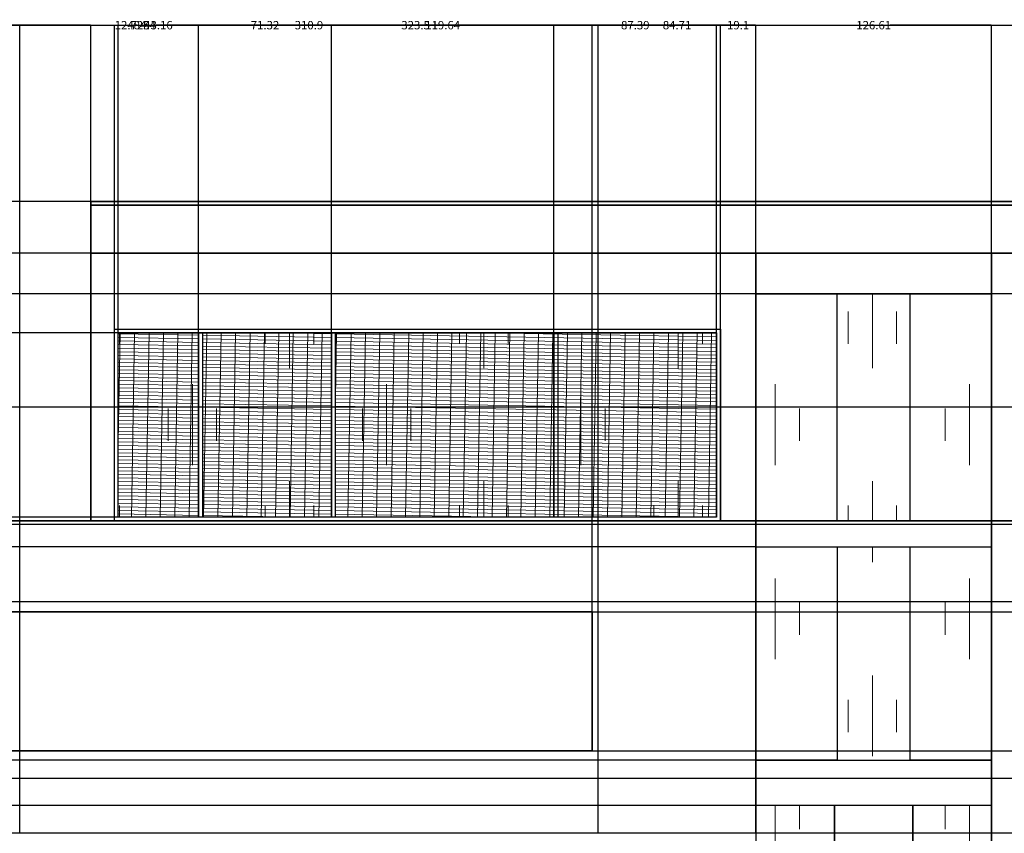
# Model space of a CAD drawing. Units: inches. Extents: x -1308 to 780, y 304 to 1023.
# Tile 4 of 7: x -667 to -138, y 585 to 1023. Entities that reach past the tile are written whole.
import ezdxf

# ---------------------------------------------------------------- set-up
doc = ezdxf.new("R2010")
doc.units = ezdxf.units.IN
doc.header["$MEASUREMENT"] = 0
for name, color, linetype, lineweight in [('A-ANNO-DIMS', 2, 'Continuous', 18), ('A-ELEV', 7, 'Continuous', 35), ('A-ELEV-PATT', 8, 'Continuous', 13), ('A-GLAZ', 4, 'Continuous', 25)]:
    doc.layers.add(name, color=color, linetype=linetype, lineweight=lineweight)
doc.styles.get("Standard").update_dxf_attribs({"font": 'arial.ttf'})
doc.dimstyles.get("Standard").update_dxf_attribs({"dimtxt": 4.5, "dimasz": 0.18, "dimexe": 0.18, "dimexo": 0.0625, "dimgap": 0.09, "dimtad": 0, "dimtih": 1, "dimtoh": 1, "dimdec": 4, "dimzin": 0, "dimdsep": 46, "dimlunit": 4, "dimtxsty": 'Standard', "dimcen": 0.09, "dimadec": 0, "dimazin": 0, "dimtfac": 1, "dimtdec": 4, "dimtofl": 0, "dimtmove": 0, "dimatfit": 3, "dimfxl": 1, "dimtolj": 1, "dimtzin": 0, "dimarcsym": 0})

# ---------------------------------------------------------------- blocks, each defined once
blk = doc.blocks.new('*D6')
at = {"layer": 'A-ANNO-DIMS', "color": 0, "lineweight": -2, "transparency": 16777216}
for p, q in [((-666.95, 585.1), (-666.95, 1019.77)), ((-666.77, 1019.59), (-519.19, 1019.59)), ((-356.24, 1019.59), (-503.82, 1019.59)), ((-356.06, 585.1), (-356.06, 1019.77))]:
    blk.add_line(p, q, dxfattribs=at)
at = {"layer": 'A-ANNO-DIMS', "color": 0, "transparency": 16777216}
for points in [[(-666.77, 1019.62), (-666.77, 1019.56), (-666.95, 1019.59)], [(-356.24, 1019.62), (-356.24, 1019.56), (-356.06, 1019.59)]]:
    blk.add_solid(points, dxfattribs=at)
at = {"layer": 'Defpoints', "color": 0, "transparency": 16777216}
for p in [(-356.06, 1019.59), (-666.95, 585.04), (-356.06, 585.04)]:
    blk.add_point(p, dxfattribs=at)
at = {"layer": 'A-ANNO-DIMS', "color": 0, "transparency": 16777216, "insert": (-511.5, 1019.59), "char_height": 4.5, "attachment_point": 5}
blk.add_mtext('\\A1;310.9', dxfattribs=at)
blk = doc.blocks.new('*D7')
at = {"layer": 'A-ANNO-DIMS', "color": 0, "lineweight": -2, "transparency": 16777216}
for p, q in [((-356.06, 585.1), (-356.06, 1019.77)), ((-355.88, 1019.59), (-320.95, 1019.59)), ((-271.53, 1019.59), (-306.45, 1019.59)), ((-271.35, 585.1), (-271.35, 1019.77))]:
    blk.add_line(p, q, dxfattribs=at)
at = {"layer": 'A-ANNO-DIMS', "color": 0, "transparency": 16777216}
for points in [[(-355.88, 1019.62), (-355.88, 1019.56), (-356.06, 1019.59)], [(-271.53, 1019.62), (-271.53, 1019.56), (-271.35, 1019.59)]]:
    blk.add_solid(points, dxfattribs=at)
at = {"layer": 'Defpoints', "color": 0, "transparency": 16777216}
for p in [(-271.35, 1019.59), (-356.06, 585.04), (-271.35, 585.04)]:
    blk.add_point(p, dxfattribs=at)
at = {"layer": 'A-ANNO-DIMS', "color": 0, "transparency": 16777216, "insert": (-313.7, 1019.59), "char_height": 4.5, "attachment_point": 5}
blk.add_mtext('\\A1;84.71', dxfattribs=at)
blk = doc.blocks.new('*D8')
at = {"layer": 'A-ANNO-DIMS', "color": 0, "lineweight": -2, "transparency": 16777216}
for p, q in [((-271.35, 585.1), (-271.35, 1019.77)), ((-271.17, 1019.59), (-216.82, 1019.59)), ((-144.91, 1019.59), (-199.25, 1019.59)), ((-144.73, 585.1), (-144.73, 1019.77))]:
    blk.add_line(p, q, dxfattribs=at)
at = {"layer": 'A-ANNO-DIMS', "color": 0, "transparency": 16777216}
for points in [[(-271.17, 1019.62), (-271.17, 1019.56), (-271.35, 1019.59)], [(-144.91, 1019.62), (-144.91, 1019.56), (-144.73, 1019.59)]]:
    blk.add_solid(points, dxfattribs=at)
at = {"layer": 'Defpoints', "color": 0, "transparency": 16777216}
for p in [(-144.73, 1019.59), (-271.35, 585.04), (-144.73, 585.04)]:
    blk.add_point(p, dxfattribs=at)
at = {"layer": 'A-ANNO-DIMS', "color": 0, "transparency": 16777216, "insert": (-208.04, 1019.59), "char_height": 4.5, "attachment_point": 5}
blk.add_mtext('\\A1;126.61', dxfattribs=at)
blk = doc.blocks.new('*D17')
at = {"layer": 'A-ANNO-DIMS', "color": 0, "lineweight": -2, "transparency": 16777216}
for p, q in [((-843.6, 753.1), (-843.6, 1019.77)), ((-843.42, 1019.59), (-743.87, 1019.59)), ((-628.86, 1019.59), (-728.41, 1019.59)), ((-628.68, 753.1), (-628.68, 1019.77))]:
    blk.add_line(p, q, dxfattribs=at)
at = {"layer": 'A-ANNO-DIMS', "color": 0, "transparency": 16777216}
for points in [[(-843.42, 1019.62), (-843.42, 1019.56), (-843.6, 1019.59)], [(-628.86, 1019.62), (-628.86, 1019.56), (-628.68, 1019.59)]]:
    blk.add_solid(points, dxfattribs=at)
at = {"layer": 'Defpoints', "color": 0, "transparency": 16777216}
for p in [(-628.68, 1019.59), (-843.6, 753.04), (-628.68, 753.04)]:
    blk.add_point(p, dxfattribs=at)
at = {"layer": 'A-ANNO-DIMS', "color": 0, "transparency": 16777216, "insert": (-736.14, 1019.59), "char_height": 4.5, "attachment_point": 5}
blk.add_mtext('\\A1;214.9', dxfattribs=at)
blk = doc.blocks.new('*D18')
at = {"layer": 'A-ANNO-DIMS', "color": 0, "lineweight": -2, "transparency": 16777216}
for p, q in [((-628.68, 924.9), (-628.68, 1019.77)), ((-628.5, 1019.59), (-60.08, 1019.59)), ((526.78, 1019.59), (-41.64, 1019.59)), ((526.96, 924.9), (526.96, 1019.77))]:
    blk.add_line(p, q, dxfattribs=at)
at = {"layer": 'A-ANNO-DIMS', "color": 0, "transparency": 16777216}
for points in [[(-628.5, 1019.62), (-628.5, 1019.56), (-628.68, 1019.59)], [(526.78, 1019.62), (526.78, 1019.56), (526.96, 1019.59)]]:
    blk.add_solid(points, dxfattribs=at)
at = {"layer": 'Defpoints', "color": 0, "transparency": 16777216}
for p in [(526.96, 1019.59), (-628.68, 924.84), (526.96, 924.84)]:
    blk.add_point(p, dxfattribs=at)
at = {"layer": 'A-ANNO-DIMS', "color": 0, "transparency": 16777216, "insert": (-50.86, 1019.59), "char_height": 4.5, "attachment_point": 5}
blk.add_mtext('\\A1;1155.6', dxfattribs=at)
blk = doc.blocks.new('*D20')
at = {"layer": 'A-ANNO-DIMS', "color": 0, "lineweight": -2, "transparency": 16777216}
for p, q in [((-615.96, 856.16), (-615.96, 1019.77)), ((-615.78, 1019.59), (-461.9, 1019.59)), ((-292.63, 1019.59), (-446.5, 1019.59)), ((-292.45, 854.16), (-292.45, 1019.77))]:
    blk.add_line(p, q, dxfattribs=at)
at = {"layer": 'A-ANNO-DIMS', "color": 0, "transparency": 16777216}
for points in [[(-615.78, 1019.62), (-615.78, 1019.56), (-615.96, 1019.59)], [(-292.63, 1019.62), (-292.63, 1019.56), (-292.45, 1019.59)]]:
    blk.add_solid(points, dxfattribs=at)
at = {"layer": 'Defpoints', "color": 0, "transparency": 16777216}
for p in [(-292.45, 1019.59), (-615.96, 856.09), (-292.45, 854.09)]:
    blk.add_point(p, dxfattribs=at)
at = {"layer": 'A-ANNO-DIMS', "color": 0, "transparency": 16777216, "insert": (-454.2, 1019.59), "char_height": 4.5, "attachment_point": 5}
blk.add_mtext('\\A1;323.5', dxfattribs=at)
blk = doc.blocks.new('*D21')
at = {"layer": 'A-ANNO-DIMS', "color": 0, "lineweight": -2, "transparency": 16777216}
for p, q in [((-628.68, 753.1), (-628.68, 1019.77)), ((-628.5, 1019.59), (-616.14, 1019.59)), ((-615.96, 753.1), (-615.96, 1019.77)), ((-615.96, 1019.59), (-615.78, 1019.59))]:
    blk.add_line(p, q, dxfattribs=at)
at = {"layer": 'A-ANNO-DIMS', "color": 0, "transparency": 16777216}
for points in [[(-628.5, 1019.62), (-628.5, 1019.56), (-628.68, 1019.59)], [(-616.14, 1019.62), (-616.14, 1019.56), (-615.96, 1019.59)]]:
    blk.add_solid(points, dxfattribs=at)
at = {"layer": 'Defpoints', "color": 0, "transparency": 16777216}
for p in [(-615.96, 1019.59), (-628.68, 753.04), (-615.96, 753.04)]:
    blk.add_point(p, dxfattribs=at)
at = {"layer": 'A-ANNO-DIMS', "color": 0, "transparency": 16777216, "insert": (-606.54, 1019.59), "char_height": 4.5, "attachment_point": 5}
blk.add_mtext('\\A1;12.725', dxfattribs=at)
blk = doc.blocks.new('*D22')
at = {"layer": 'A-ANNO-DIMS', "color": 0, "lineweight": -2, "transparency": 16777216}
for p, q in [((-290.45, 753.1), (-290.45, 1019.77)), ((-290.27, 1019.59), (-286.18, 1019.59)), ((-271.53, 1019.59), (-275.61, 1019.59)), ((-271.35, 753.1), (-271.35, 1019.77))]:
    blk.add_line(p, q, dxfattribs=at)
at = {"layer": 'A-ANNO-DIMS', "color": 0, "transparency": 16777216}
for points in [[(-290.27, 1019.62), (-290.27, 1019.56), (-290.45, 1019.59)], [(-271.53, 1019.62), (-271.53, 1019.56), (-271.35, 1019.59)]]:
    blk.add_solid(points, dxfattribs=at)
at = {"layer": 'Defpoints', "color": 0, "transparency": 16777216}
for p in [(-271.35, 1019.59), (-290.45, 753.04), (-271.35, 753.04)]:
    blk.add_point(p, dxfattribs=at)
at = {"layer": 'A-ANNO-DIMS', "color": 0, "transparency": 16777216, "insert": (-280.9, 1019.59), "char_height": 4.5, "attachment_point": 5}
blk.add_mtext('\\A1;19.1', dxfattribs=at)
blk = doc.blocks.new('*D23')
at = {"layer": 'A-ANNO-DIMS', "color": 0, "lineweight": -2, "transparency": 16777216}
for p, q in [((-613.96, 755.1), (-613.96, 1019.77)), ((-613.78, 1019.59), (-600.15, 1019.59)), ((-570.98, 1019.59), (-584.6, 1019.59)), ((-570.8, 755.1), (-570.8, 1019.77))]:
    blk.add_line(p, q, dxfattribs=at)
at = {"layer": 'A-ANNO-DIMS', "color": 0, "transparency": 16777216}
for points in [[(-613.78, 1019.62), (-613.78, 1019.56), (-613.96, 1019.59)], [(-570.98, 1019.62), (-570.98, 1019.56), (-570.8, 1019.59)]]:
    blk.add_solid(points, dxfattribs=at)
at = {"layer": 'Defpoints', "color": 0, "transparency": 16777216}
for p in [(-570.8, 1019.59), (-613.96, 755.04), (-570.8, 755.04)]:
    blk.add_point(p, dxfattribs=at)
at = {"layer": 'A-ANNO-DIMS', "color": 0, "transparency": 16777216, "insert": (-592.38, 1019.59), "char_height": 4.5, "attachment_point": 5}
blk.add_mtext('\\A1;43.16', dxfattribs=at)
blk = doc.blocks.new('*D24')
at = {"layer": 'A-ANNO-DIMS', "color": 0, "lineweight": -2, "transparency": 16777216}
for p, q in [((-570.8, 755.1), (-570.8, 1019.77)), ((-570.62, 1019.59), (-542.78, 1019.59)), ((-499.65, 1019.59), (-527.49, 1019.59)), ((-499.47, 755.1), (-499.47, 1019.77))]:
    blk.add_line(p, q, dxfattribs=at)
at = {"layer": 'A-ANNO-DIMS', "color": 0, "transparency": 16777216}
for points in [[(-570.62, 1019.62), (-570.62, 1019.56), (-570.8, 1019.59)], [(-499.65, 1019.62), (-499.65, 1019.56), (-499.47, 1019.59)]]:
    blk.add_solid(points, dxfattribs=at)
at = {"layer": 'Defpoints', "color": 0, "transparency": 16777216}
for p in [(-499.47, 1019.59), (-570.8, 755.04), (-499.47, 755.04)]:
    blk.add_point(p, dxfattribs=at)
at = {"layer": 'A-ANNO-DIMS', "color": 0, "transparency": 16777216, "insert": (-535.13, 1019.59), "char_height": 4.5, "attachment_point": 5}
blk.add_mtext('\\A1;71.32', dxfattribs=at)
blk = doc.blocks.new('*D25')
at = {"layer": 'A-ANNO-DIMS', "color": 0, "lineweight": -2, "transparency": 16777216}
for p, q in [((-499.47, 755.1), (-499.47, 1019.77)), ((-499.29, 1019.59), (-448.86, 1019.59)), ((-380.02, 1019.59), (-430.45, 1019.59)), ((-379.84, 755.1), (-379.84, 1019.77))]:
    blk.add_line(p, q, dxfattribs=at)
at = {"layer": 'A-ANNO-DIMS', "color": 0, "transparency": 16777216}
for points in [[(-499.29, 1019.62), (-499.29, 1019.56), (-499.47, 1019.59)], [(-380.02, 1019.62), (-380.02, 1019.56), (-379.84, 1019.59)]]:
    blk.add_solid(points, dxfattribs=at)
at = {"layer": 'Defpoints', "color": 0, "transparency": 16777216}
for p in [(-379.84, 1019.59), (-499.47, 755.04), (-379.84, 755.04)]:
    blk.add_point(p, dxfattribs=at)
at = {"layer": 'A-ANNO-DIMS', "color": 0, "transparency": 16777216, "insert": (-439.65, 1019.59), "char_height": 4.5, "attachment_point": 5}
blk.add_mtext('\\A1;119.64', dxfattribs=at)
blk = doc.blocks.new('*D26')
at = {"layer": 'A-ANNO-DIMS', "color": 0, "lineweight": -2, "transparency": 16777216}
for p, q in [((-379.84, 755.1), (-379.84, 1019.77)), ((-379.66, 1019.59), (-343.83, 1019.59)), ((-292.63, 1019.59), (-328.45, 1019.59)), ((-292.45, 755.1), (-292.45, 1019.77))]:
    blk.add_line(p, q, dxfattribs=at)
at = {"layer": 'A-ANNO-DIMS', "color": 0, "transparency": 16777216}
for points in [[(-379.66, 1019.62), (-379.66, 1019.56), (-379.84, 1019.59)], [(-292.63, 1019.62), (-292.63, 1019.56), (-292.45, 1019.59)]]:
    blk.add_solid(points, dxfattribs=at)
at = {"layer": 'Defpoints', "color": 0, "transparency": 16777216}
for p in [(-292.45, 1019.59), (-379.84, 755.04), (-292.45, 755.04)]:
    blk.add_point(p, dxfattribs=at)
at = {"layer": 'A-ANNO-DIMS', "color": 0, "transparency": 16777216, "insert": (-336.14, 1019.59), "char_height": 4.5, "attachment_point": 5}
blk.add_mtext('\\A1;87.39', dxfattribs=at)
blk = doc.blocks.new('*D27')
at = {"layer": 'A-ANNO-DIMS', "color": 0, "lineweight": -2, "transparency": 16777216}
for p, q in [((-144.73, 753.1), (-144.73, 1019.77)), ((-144.55, 1019.59), (-112.53, 1019.59)), ((-65.19, 1019.59), (-97.21, 1019.59)), ((-65.01, 751.1), (-65.01, 1019.77))]:
    blk.add_line(p, q, dxfattribs=at)
at = {"layer": 'A-ANNO-DIMS', "color": 0, "transparency": 16777216}
for points in [[(-144.55, 1019.62), (-144.55, 1019.56), (-144.73, 1019.59)], [(-65.19, 1019.62), (-65.19, 1019.56), (-65.01, 1019.59)]]:
    blk.add_solid(points, dxfattribs=at)
at = {"layer": 'Defpoints', "color": 0, "transparency": 16777216}
for p in [(-65.01, 1019.59), (-144.73, 753.04), (-65.01, 751.04)]:
    blk.add_point(p, dxfattribs=at)
at = {"layer": 'A-ANNO-DIMS', "color": 0, "transparency": 16777216, "insert": (-104.87, 1019.59), "char_height": 4.5, "attachment_point": 5}
blk.add_mtext('\\A1;79.73', dxfattribs=at)
blk = doc.blocks.new('*D45')
at = {"layer": 'A-ANNO-DIMS', "color": 0, "lineweight": -2, "transparency": 16777216}
for p, q in [((-25.86, 614.44), (-25.86, 307.09)), ((-144.73, 584.98), (-144.73, 307.09)), ((-144.55, 307.27), (-94.52, 307.27)), ((-26.04, 307.27), (-76.07, 307.27))]:
    blk.add_line(p, q, dxfattribs=at)
at = {"layer": 'A-ANNO-DIMS', "color": 0, "transparency": 16777216}
for points in [[(-144.55, 307.3), (-144.55, 307.24), (-144.73, 307.27)], [(-26.04, 307.3), (-26.04, 307.24), (-25.86, 307.27)]]:
    blk.add_solid(points, dxfattribs=at)
at = {"layer": 'Defpoints', "color": 0, "transparency": 16777216}
for p in [(-25.86, 614.51), (-144.73, 585.04), (-25.86, 307.27)]:
    blk.add_point(p, dxfattribs=at)
at = {"layer": 'A-ANNO-DIMS', "color": 0, "transparency": 16777216, "insert": (-85.3, 307.27), "char_height": 4.5, "attachment_point": 5}
blk.add_mtext('\\A1;118.88', dxfattribs=at)
blk = doc.blocks.new('*D48')
at = {"layer": 'A-ANNO-DIMS', "color": 0, "lineweight": -2, "transparency": 16777216}
for p, q in [((-843.6, 704.15), (-843.6, 1019.77)), ((-843.42, 1019.59), (-609.19, 1019.59)), ((-359.42, 1019.59), (-593.66, 1019.59)), ((-359.24, 704.15), (-359.24, 1019.77))]:
    blk.add_line(p, q, dxfattribs=at)
at = {"layer": 'A-ANNO-DIMS', "color": 0, "transparency": 16777216}
for points in [[(-843.42, 1019.62), (-843.42, 1019.56), (-843.6, 1019.59)], [(-359.42, 1019.62), (-359.42, 1019.56), (-359.24, 1019.59)]]:
    blk.add_solid(points, dxfattribs=at)
at = {"layer": 'Defpoints', "color": 0, "transparency": 16777216}
for p in [(-359.24, 1019.59), (-843.6, 704.09), (-359.24, 704.09)]:
    blk.add_point(p, dxfattribs=at)
at = {"layer": 'A-ANNO-DIMS', "color": 0, "transparency": 16777216, "insert": (-601.42, 1019.59), "char_height": 4.5, "attachment_point": 5}
blk.add_mtext('\\A1;484.4', dxfattribs=at)
blk = doc.blocks.new('*D57')
at = {"layer": 'A-ANNO-DIMS', "color": 0, "lineweight": -2, "transparency": 16777216}
for p, q in [((-628.74, 924.84), (-1298.45, 924.84)), ((-1298.27, 924.66), (-1298.27, 665.82)), ((-1298.27, 402.2), (-1298.27, 661.04)), ((-1203.58, 402.02), (-1298.45, 402.02))]:
    blk.add_line(p, q, dxfattribs=at)
at = {"layer": 'A-ANNO-DIMS', "color": 0, "transparency": 16777216}
for points in [[(-1298.3, 924.66), (-1298.24, 924.66), (-1298.27, 924.84)], [(-1298.3, 402.2), (-1298.24, 402.2), (-1298.27, 402.02)]]:
    blk.add_solid(points, dxfattribs=at)
at = {"layer": 'Defpoints', "color": 0, "transparency": 16777216}
for p in [(-1298.27, 924.84), (-628.68, 924.84), (-1203.52, 402.02)]:
    blk.add_point(p, dxfattribs=at)
at = {"layer": 'A-ANNO-DIMS', "color": 0, "transparency": 16777216, "insert": (-1298.27, 663.43), "char_height": 4.5, "attachment_point": 5}
blk.add_mtext('\\A1;522.8', dxfattribs=at)
blk = doc.blocks.new('*D63')
at = {"layer": 'A-ANNO-DIMS', "color": 0, "lineweight": -2, "transparency": 16777216}
for p, q in [((-843.54, 629.44), (771.09, 629.44)), ((770.91, 629.26), (770.91, 518.12)), ((770.91, 402.2), (770.91, 513.34)), ((-843.54, 402.02), (771.09, 402.02))]:
    blk.add_line(p, q, dxfattribs=at)
at = {"layer": 'A-ANNO-DIMS', "color": 0, "transparency": 16777216}
for points in [[(770.88, 629.26), (770.94, 629.26), (770.91, 629.44)], [(770.88, 402.2), (770.94, 402.2), (770.91, 402.02)]]:
    blk.add_solid(points, dxfattribs=at)
at = {"layer": 'Defpoints', "color": 0, "transparency": 16777216}
for p in [(-843.6, 629.44), (770.91, 629.44), (-843.6, 402.02)]:
    blk.add_point(p, dxfattribs=at)
at = {"layer": 'A-ANNO-DIMS', "color": 0, "transparency": 16777216, "insert": (770.91, 515.73), "char_height": 4.5, "attachment_point": 5}
blk.add_mtext('\\A1;227.43', dxfattribs=at)
blk = doc.blocks.new('*D64')
at = {"layer": 'A-ANNO-DIMS', "color": 0, "lineweight": -2, "transparency": 16777216}
for p, q in [((-843.54, 704.09), (771.09, 704.09)), ((770.91, 703.91), (770.91, 669.15)), ((770.91, 629.62), (770.91, 664.38)), ((-843.54, 629.44), (771.09, 629.44))]:
    blk.add_line(p, q, dxfattribs=at)
at = {"layer": 'A-ANNO-DIMS', "color": 0, "transparency": 16777216}
for points in [[(770.88, 703.91), (770.94, 703.91), (770.91, 704.09)], [(770.88, 629.62), (770.94, 629.62), (770.91, 629.44)]]:
    blk.add_solid(points, dxfattribs=at)
at = {"layer": 'Defpoints', "color": 0, "transparency": 16777216}
for p in [(-843.6, 704.09), (770.91, 704.09), (-843.6, 629.44)]:
    blk.add_point(p, dxfattribs=at)
at = {"layer": 'A-ANNO-DIMS', "color": 0, "transparency": 16777216, "insert": (770.91, 666.76), "char_height": 4.5, "attachment_point": 5}
blk.add_mtext('\\A1;74.64', dxfattribs=at)
blk = doc.blocks.new('*D65')
at = {"layer": 'A-ANNO-DIMS', "color": 0, "lineweight": -2, "transparency": 16777216}
for p, q in [((-843.54, 753.04), (771.09, 753.04)), ((770.91, 752.86), (770.91, 730.95)), ((770.91, 704.27), (770.91, 726.17)), ((-843.54, 704.09), (771.09, 704.09))]:
    blk.add_line(p, q, dxfattribs=at)
at = {"layer": 'A-ANNO-DIMS', "color": 0, "transparency": 16777216}
for points in [[(770.88, 752.86), (770.94, 752.86), (770.91, 753.04)], [(770.88, 704.27), (770.94, 704.27), (770.91, 704.09)]]:
    blk.add_solid(points, dxfattribs=at)
at = {"layer": 'Defpoints', "color": 0, "transparency": 16777216}
for p in [(-843.6, 753.04), (770.91, 753.04), (-843.6, 704.09)]:
    blk.add_point(p, dxfattribs=at)
at = {"layer": 'A-ANNO-DIMS', "color": 0, "transparency": 16777216, "insert": (770.91, 728.56), "char_height": 4.5, "attachment_point": 5}
blk.add_mtext('\\A1;48.95', dxfattribs=at)
blk = doc.blocks.new('*D67')
at = {"layer": 'A-ANNO-DIMS', "color": 0, "lineweight": -2, "transparency": 16777216}
for p, q in [((-271.41, 600.04), (-1298.45, 600.04)), ((-1298.27, 599.86), (-1298.27, 507.96)), ((-1298.27, 411.28), (-1298.27, 503.18)), ((-271.41, 411.1), (-1298.45, 411.1))]:
    blk.add_line(p, q, dxfattribs=at)
at = {"layer": 'A-ANNO-DIMS', "color": 0, "transparency": 16777216}
for points in [[(-1298.3, 599.86), (-1298.24, 599.86), (-1298.27, 600.04)], [(-1298.3, 411.28), (-1298.24, 411.28), (-1298.27, 411.1)]]:
    blk.add_solid(points, dxfattribs=at)
at = {"layer": 'Defpoints', "color": 0, "transparency": 16777216}
for p in [(-1298.27, 600.04), (-271.35, 600.04), (-271.35, 411.1)]:
    blk.add_point(p, dxfattribs=at)
at = {"layer": 'A-ANNO-DIMS', "color": 0, "transparency": 16777216, "insert": (-1298.27, 505.57), "char_height": 4.5, "attachment_point": 5}
blk.add_mtext('\\A1;188.94', dxfattribs=at)
blk = doc.blocks.new('*D68')
at = {"layer": 'A-ANNO-DIMS', "color": 0, "lineweight": -2, "transparency": 16777216}
for p, q in [((-271.41, 624.44), (-1298.45, 624.44)), ((-1298.27, 624.26), (-1298.27, 614.59)), ((-1298.27, 600.22), (-1298.27, 609.89)), ((-271.41, 600.04), (-1298.45, 600.04))]:
    blk.add_line(p, q, dxfattribs=at)
at = {"layer": 'A-ANNO-DIMS', "color": 0, "transparency": 16777216}
for points in [[(-1298.3, 624.26), (-1298.24, 624.26), (-1298.27, 624.44)], [(-1298.3, 600.22), (-1298.24, 600.22), (-1298.27, 600.04)]]:
    blk.add_solid(points, dxfattribs=at)
at = {"layer": 'Defpoints', "color": 0, "transparency": 16777216}
for p in [(-1298.27, 624.44), (-271.35, 624.44), (-271.35, 600.04)]:
    blk.add_point(p, dxfattribs=at)
at = {"layer": 'A-ANNO-DIMS', "color": 0, "transparency": 16777216, "insert": (-1298.27, 612.24), "char_height": 4.5, "attachment_point": 5}
blk.add_mtext('\\A1;24.4', dxfattribs=at)
blk = doc.blocks.new('*D69')
at = {"layer": 'A-ANNO-DIMS', "color": 0, "lineweight": -2, "transparency": 16777216}
for p, q in [((-271.41, 739.03), (-1298.45, 739.03)), ((-1298.27, 738.85), (-1298.27, 684.12)), ((-1298.27, 624.62), (-1298.27, 679.35)), ((-271.41, 624.44), (-1298.45, 624.44))]:
    blk.add_line(p, q, dxfattribs=at)
at = {"layer": 'A-ANNO-DIMS', "color": 0, "transparency": 16777216}
for points in [[(-1298.3, 738.85), (-1298.24, 738.85), (-1298.27, 739.03)], [(-1298.3, 624.62), (-1298.24, 624.62), (-1298.27, 624.44)]]:
    blk.add_solid(points, dxfattribs=at)
at = {"layer": 'Defpoints', "color": 0, "transparency": 16777216}
for p in [(-1298.27, 739.03), (-271.35, 739.03), (-271.35, 624.44)]:
    blk.add_point(p, dxfattribs=at)
at = {"layer": 'A-ANNO-DIMS', "color": 0, "transparency": 16777216, "insert": (-1298.27, 681.73), "char_height": 4.5, "attachment_point": 5}
blk.add_mtext('\\A1;114.58', dxfattribs=at)
blk = doc.blocks.new('*D70')
at = {"layer": 'A-ANNO-DIMS', "color": 0, "lineweight": -2, "transparency": 16777216}
for p, q in [((-271.41, 753.04), (-1298.45, 753.04)), ((-1298.27, 752.86), (-1298.27, 748.42)), ((-1298.27, 739.21), (-1298.27, 743.64)), ((-271.41, 739.03), (-1298.45, 739.03))]:
    blk.add_line(p, q, dxfattribs=at)
at = {"layer": 'A-ANNO-DIMS', "color": 0, "transparency": 16777216}
for points in [[(-1298.3, 752.86), (-1298.24, 752.86), (-1298.27, 753.04)], [(-1298.3, 739.21), (-1298.24, 739.21), (-1298.27, 739.03)]]:
    blk.add_solid(points, dxfattribs=at)
at = {"layer": 'Defpoints', "color": 0, "transparency": 16777216}
for p in [(-1298.27, 753.04), (-271.35, 753.04), (-271.35, 739.03)]:
    blk.add_point(p, dxfattribs=at)
at = {"layer": 'A-ANNO-DIMS', "color": 0, "transparency": 16777216, "insert": (-1298.27, 746.03), "char_height": 4.5, "attachment_point": 5}
blk.add_mtext('\\A1;14.013', dxfattribs=at)
blk = doc.blocks.new('*D71')
at = {"layer": 'A-ANNO-DIMS', "color": 0, "lineweight": -2, "transparency": 16777216}
for p, q in [((-271.41, 875.17), (-1298.45, 875.17)), ((-1298.27, 874.99), (-1298.27, 816.49)), ((-1298.27, 753.22), (-1298.27, 811.72)), ((-271.41, 753.04), (-1298.45, 753.04))]:
    blk.add_line(p, q, dxfattribs=at)
at = {"layer": 'A-ANNO-DIMS', "color": 0, "transparency": 16777216}
for points in [[(-1298.3, 874.99), (-1298.24, 874.99), (-1298.27, 875.17)], [(-1298.3, 753.22), (-1298.24, 753.22), (-1298.27, 753.04)]]:
    blk.add_solid(points, dxfattribs=at)
at = {"layer": 'Defpoints', "color": 0, "transparency": 16777216}
for p in [(-1298.27, 875.17), (-271.35, 875.17), (-271.35, 753.04)]:
    blk.add_point(p, dxfattribs=at)
at = {"layer": 'A-ANNO-DIMS', "color": 0, "transparency": 16777216, "insert": (-1298.27, 814.1), "char_height": 4.5, "attachment_point": 5}
blk.add_mtext('\\A1;122.13', dxfattribs=at)
blk = doc.blocks.new('*D72')
at = {"layer": 'A-ANNO-DIMS', "color": 0, "lineweight": -2, "transparency": 16777216}
for p, q in [((-271.41, 897.04), (-1298.45, 897.04)), ((-1298.27, 896.86), (-1298.27, 888.49)), ((-1298.27, 875.35), (-1298.27, 883.72)), ((-271.41, 875.17), (-1298.45, 875.17))]:
    blk.add_line(p, q, dxfattribs=at)
at = {"layer": 'A-ANNO-DIMS', "color": 0, "transparency": 16777216}
for points in [[(-1298.3, 896.86), (-1298.24, 896.86), (-1298.27, 897.04)], [(-1298.3, 875.35), (-1298.24, 875.35), (-1298.27, 875.17)]]:
    blk.add_solid(points, dxfattribs=at)
at = {"layer": 'Defpoints', "color": 0, "transparency": 16777216}
for p in [(-1298.27, 897.04), (-271.35, 897.04), (-271.35, 875.17)]:
    blk.add_point(p, dxfattribs=at)
at = {"layer": 'A-ANNO-DIMS', "color": 0, "transparency": 16777216, "insert": (-1298.27, 886.1), "char_height": 4.5, "attachment_point": 5}
blk.add_mtext('\\A1;21.868', dxfattribs=at)
blk = doc.blocks.new('*D81')
at = {"layer": 'A-ANNO-DIMS', "color": 0, "lineweight": -2, "transparency": 16777216}
for p, q in [((-25.92, 614.51), (-1298.45, 614.51)), ((-1298.27, 614.33), (-1298.27, 602.16)), ((-1298.27, 585.22), (-1298.27, 597.39)), ((-59.22, 585.04), (-1298.45, 585.04))]:
    blk.add_line(p, q, dxfattribs=at)
at = {"layer": 'A-ANNO-DIMS', "color": 0, "transparency": 16777216}
for points in [[(-1298.3, 614.33), (-1298.24, 614.33), (-1298.27, 614.51)], [(-1298.3, 585.22), (-1298.24, 585.22), (-1298.27, 585.04)]]:
    blk.add_solid(points, dxfattribs=at)
at = {"layer": 'Defpoints', "color": 0, "transparency": 16777216}
for p in [(-1298.27, 614.51), (-25.86, 614.51), (-59.16, 585.04)]:
    blk.add_point(p, dxfattribs=at)
at = {"layer": 'A-ANNO-DIMS', "color": 0, "transparency": 16777216, "insert": (-1298.27, 599.77), "char_height": 4.5, "attachment_point": 5}
blk.add_mtext('\\A1;29.47', dxfattribs=at)
blk = doc.blocks.new('*D82')
at = {"layer": 'A-ANNO-DIMS', "color": 0, "lineweight": -2, "transparency": 16777216}
for p, q in [((-25.92, 709.46), (-1298.45, 709.46)), ((-1298.27, 709.28), (-1298.27, 664.37)), ((-1298.27, 614.69), (-1298.27, 659.6)), ((-25.92, 614.51), (-1298.45, 614.51))]:
    blk.add_line(p, q, dxfattribs=at)
at = {"layer": 'A-ANNO-DIMS', "color": 0, "transparency": 16777216}
for points in [[(-1298.3, 709.28), (-1298.24, 709.28), (-1298.27, 709.46)], [(-1298.3, 614.69), (-1298.24, 614.69), (-1298.27, 614.51)]]:
    blk.add_solid(points, dxfattribs=at)
at = {"layer": 'Defpoints', "color": 0, "transparency": 16777216}
for p in [(-1298.27, 709.46), (-25.86, 709.46), (-25.86, 614.51)]:
    blk.add_point(p, dxfattribs=at)
at = {"layer": 'A-ANNO-DIMS', "color": 0, "transparency": 16777216, "insert": (-1298.27, 661.98), "char_height": 4.5, "attachment_point": 5}
blk.add_mtext('\\A1;94.95', dxfattribs=at)
blk = doc.blocks.new('*D83')
at = {"layer": 'A-ANNO-DIMS', "color": 0, "lineweight": -2, "transparency": 16777216}
for p, q in [((4.02, 753.04), (-1298.45, 753.04)), ((-1298.27, 752.86), (-1298.27, 733.64)), ((-1298.27, 709.64), (-1298.27, 728.86)), ((-25.92, 709.46), (-1298.45, 709.46))]:
    blk.add_line(p, q, dxfattribs=at)
at = {"layer": 'A-ANNO-DIMS', "color": 0, "transparency": 16777216}
for points in [[(-1298.3, 752.86), (-1298.24, 752.86), (-1298.27, 753.04)], [(-1298.3, 709.64), (-1298.24, 709.64), (-1298.27, 709.46)]]:
    blk.add_solid(points, dxfattribs=at)
at = {"layer": 'Defpoints', "color": 0, "transparency": 16777216}
for p in [(-1298.27, 753.04), (4.08, 753.04), (-25.86, 709.46)]:
    blk.add_point(p, dxfattribs=at)
at = {"layer": 'A-ANNO-DIMS', "color": 0, "transparency": 16777216, "insert": (-1298.27, 731.25), "char_height": 4.5, "attachment_point": 5}
blk.add_mtext('\\A1;43.58', dxfattribs=at)
blk = doc.blocks.new('*D84')
at = {"layer": 'A-ANNO-DIMS', "color": 0, "lineweight": -2, "transparency": 16777216}
for p, q in [((-292.51, 854.09), (-1298.45, 854.09)), ((-1298.27, 853.91), (-1298.27, 806.95)), ((-1298.27, 755.22), (-1298.27, 802.18)), ((-292.51, 755.04), (-1298.45, 755.04))]:
    blk.add_line(p, q, dxfattribs=at)
at = {"layer": 'A-ANNO-DIMS', "color": 0, "transparency": 16777216}
for points in [[(-1298.3, 853.91), (-1298.24, 853.91), (-1298.27, 854.09)], [(-1298.3, 755.22), (-1298.24, 755.22), (-1298.27, 755.04)]]:
    blk.add_solid(points, dxfattribs=at)
at = {"layer": 'Defpoints', "color": 0, "transparency": 16777216}
for p in [(-1298.27, 854.09), (-292.45, 854.09), (-292.45, 755.04)]:
    blk.add_point(p, dxfattribs=at)
at = {"layer": 'A-ANNO-DIMS', "color": 0, "transparency": 16777216, "insert": (-1298.27, 804.57), "char_height": 4.5, "attachment_point": 5}
blk.add_mtext('\\A1;99.06', dxfattribs=at)
blk = doc.blocks.new('*D85')
at = {"layer": 'A-ANNO-DIMS', "color": 0, "lineweight": -2, "transparency": 16777216}
for p, q in [((-63.07, 875.17), (-1298.45, 875.17)), ((-1298.27, 874.99), (-1298.27, 815.49)), ((-1298.27, 751.22), (-1298.27, 810.72)), ((-65.07, 751.04), (-1298.45, 751.04))]:
    blk.add_line(p, q, dxfattribs=at)
at = {"layer": 'A-ANNO-DIMS', "color": 0, "transparency": 16777216}
for points in [[(-1298.3, 874.99), (-1298.24, 874.99), (-1298.27, 875.17)], [(-1298.3, 751.22), (-1298.24, 751.22), (-1298.27, 751.04)]]:
    blk.add_solid(points, dxfattribs=at)
at = {"layer": 'Defpoints', "color": 0, "transparency": 16777216}
for p in [(-1298.27, 875.17), (-63.01, 875.17), (-65.01, 751.04)]:
    blk.add_point(p, dxfattribs=at)
at = {"layer": 'A-ANNO-DIMS', "color": 0, "transparency": 16777216, "insert": (-1298.27, 813.1), "char_height": 4.5, "attachment_point": 5}
blk.add_mtext('\\A1;124.13', dxfattribs=at)
blk = doc.blocks.new('*D86')
at = {"layer": 'A-ANNO-DIMS', "color": 0, "lineweight": -2, "transparency": 16777216}
for p, q in [((79.34, 814.1), (-1298.45, 814.1)), ((-1298.27, 813.92), (-1298.27, 785.96)), ((-1298.27, 753.22), (-1298.27, 781.18)), ((79.34, 753.04), (-1298.45, 753.04))]:
    blk.add_line(p, q, dxfattribs=at)
at = {"layer": 'A-ANNO-DIMS', "color": 0, "transparency": 16777216}
for points in [[(-1298.3, 813.92), (-1298.24, 813.92), (-1298.27, 814.1)], [(-1298.3, 753.22), (-1298.24, 753.22), (-1298.27, 753.04)]]:
    blk.add_solid(points, dxfattribs=at)
at = {"layer": 'Defpoints', "color": 0, "transparency": 16777216}
for p in [(-1298.27, 814.1), (79.41, 814.1), (79.41, 753.04)]:
    blk.add_point(p, dxfattribs=at)
at = {"layer": 'A-ANNO-DIMS', "color": 0, "transparency": 16777216, "insert": (-1298.27, 783.57), "char_height": 4.5, "attachment_point": 5}
blk.add_mtext('\\A1;61.07', dxfattribs=at)
blk = doc.blocks.new('*D87')
at = {"layer": 'A-ANNO-DIMS', "color": 0, "lineweight": -2, "transparency": 16777216}
for p, q in [((110.86, 875.17), (-1298.45, 875.17)), ((-1298.27, 874.99), (-1298.27, 847.03)), ((-1298.27, 814.28), (-1298.27, 842.25)), ((79.34, 814.1), (-1298.45, 814.1))]:
    blk.add_line(p, q, dxfattribs=at)
at = {"layer": 'A-ANNO-DIMS', "color": 0, "transparency": 16777216}
for points in [[(-1298.3, 874.99), (-1298.24, 874.99), (-1298.27, 875.17)], [(-1298.3, 814.28), (-1298.24, 814.28), (-1298.27, 814.1)]]:
    blk.add_solid(points, dxfattribs=at)
at = {"layer": 'Defpoints', "color": 0, "transparency": 16777216}
for p in [(-1298.27, 875.17), (110.92, 875.17), (79.41, 814.1)]:
    blk.add_point(p, dxfattribs=at)
at = {"layer": 'A-ANNO-DIMS', "color": 0, "transparency": 16777216, "insert": (-1298.27, 844.64), "char_height": 4.5, "attachment_point": 5}
blk.add_mtext('\\A1;61.07', dxfattribs=at)

msp = doc.modelspace()

# ---------------------------------------------------------------- hatches: boundary and pattern name
at = {"layer": 'A-ELEV-PATT'}
h = msp.add_hatch(dxfattribs=at)
h.set_pattern_fill('GOST_GLASS', color=256, scale=8.7, angle=45)
h.set_pattern_definition([(90, (0, 0), (52.2, 52.2), [43.5, -60.9]), (90, (13.05, 13.05), (52.2, 52.2), [17.4, -87]), (90, (-13.05, 13.05), (52.2, 52.2), [17.4, -87])])
h.paths.add_polyline_path([(-570.795, 854.0948), (-613.9558, 854.0948), (-613.9558, 755.0385), (-570.795, 755.0385)])
h.paths.add_polyline_path([(-499.4748, 854.0948), (-568.795, 854.0948), (-568.795, 755.0385), (-499.4748, 755.0385)])
h.paths.add_polyline_path([(-379.8352, 854.0948), (-497.4748, 854.0948), (-497.4748, 755.0385), (-379.8352, 755.0385)])
h.paths.add_polyline_path([(-292.4461, 854.0948), (-377.8352, 854.0948), (-377.8352, 755.0385), (-292.4461, 755.0385)])
h.paths.add_polyline_path([(4.0783, 875.1709), (-63.0069, 875.1709), (-63.0069, 753.0385), (4.0783, 753.0385)])
h.paths.add_polyline_path([(77.4055, 875.1709), (6.0783, 875.1709), (6.0783, 753.0385), (77.4055, 753.0385)])
h.paths.add_polyline_path([(150.9148, 814.1047), (79.4055, 814.1047), (79.4055, 753.0385), (150.9148, 753.0385)])
h.paths.add_polyline_path([(110.9181, 875.1709), (79.4055, 875.1709), (79.4055, 814.1047)])
h.paths.add_polyline_path([(150.9148, 875.1709), (110.9181, 875.1709), (149.6048, 816.1047), (150.9148, 816.1047)])
h.paths.add_polyline_path([(-227.6882, 875.1709), (-271.346, 875.1709), (-271.346, 753.0385), (-227.6882, 753.0385)])
h.paths.add_polyline_path([(-188.3907, 875.1709), (-227.6882, 875.1709), (-227.6882, 753.0385), (-188.3907, 753.0385)])
h.paths.add_polyline_path([(-144.7329, 875.1709), (-188.3907, 875.1709), (-188.3907, 753.0385), (-144.7329, 753.0385)])
h.paths.add_polyline_path([(-144.7329, 739.0259), (-188.3907, 739.0259), (-188.3907, 624.4429), (-144.7329, 624.4429)])
h.paths.add_polyline_path([(-188.3907, 739.0259), (-227.6882, 739.0259), (-227.6882, 624.4429), (-188.3907, 624.4429)])
h.paths.add_polyline_path([(-227.6882, 739.0259), (-271.346, 739.0259), (-271.346, 624.4429), (-227.6882, 624.4429)])
h.paths.add_polyline_path([(-229.1416, 600.0434), (-271.346, 600.0434), (-271.346, 411.1006), (-229.1416, 411.1006)])
h.paths.add_polyline_path([(-186.9373, 600.0434), (-229.1416, 600.0434), (-229.1416, 411.1006), (-186.9373, 411.1006)])
h.paths.add_polyline_path([(-144.7329, 600.0434), (-186.9373, 600.0434), (-186.9373, 411.1006), (-144.7329, 411.1006)])
h = msp.add_hatch(dxfattribs=at)
h.set_pattern_fill('GRATE', color=256, scale=62, angle=179)
h.paths.add_polyline_path([(-499.4748, 854.0948), (-568.795, 854.0948), (-568.795, 755.0385), (-499.4748, 755.0385)])
h.paths.add_polyline_path([(-570.795, 854.0948), (-613.9558, 854.0948), (-613.9558, 755.0385), (-570.795, 755.0385)])
h.paths.add_polyline_path([(-379.8352, 854.0948), (-497.4748, 854.0948), (-497.4748, 755.0385), (-379.8352, 755.0385)])
h.paths.add_polyline_path([(-292.4461, 854.0948), (-379.8352, 854.0948), (-379.8352, 755.0385), (-292.4461, 755.0385)])

# ---------------------------------------------------------------- linework, layer by layer
at = {"layer": 'A-ELEV'}
for p, q in [((-628.6809, 924.8421), (381.6743, 924.8421)), ((-628.6809, 924.8421), (-628.6809, 922.8421)), ((-628.6809, 897.0385), (-628.6809, 922.8421)), ((-628.6809, 922.8421), (381.6743, 922.8421)), ((-628.6809, 753.0385), (-628.6809, 897.0385)), ((-628.6809, 897.0385), (-271.346, 897.0385)), ((-271.346, 753.0385), (-271.346, 897.0385)), ((-271.346, 897.0385), (-144.7329, 897.0385)), ((-144.7329, 753.0385), (-144.7329, 897.0385)), ((-130.9821, 897.0385), (-144.7329, 897.0385)), ((-843.5988, 753.0385), (-628.6809, 753.0385)), ((-271.346, 753.0385), (-628.6809, 753.0385)), ((-271.346, 600.0434), (-271.346, 753.0385)), ((-271.346, 753.0385), (-144.7329, 753.0385)), ((526.9606, 753.0385), (-144.7329, 753.0385)), ((-144.7329, 753.0385), (-144.7329, 585.0385)), ((-359.2437, 704.0857), (-843.5988, 704.0857)), ((-359.2437, 629.4421), (-359.2437, 704.0857)), ((-843.5988, 629.4421), (-390.5363, 629.4421)), ((-390.5363, 629.4421), (-359.2437, 629.4421))]:
    msp.add_line(p, q, dxfattribs=at)
at = {"layer": 'A-GLAZ'}
for p, q in [((-271.346, 875.1709), (-144.7329, 875.1709)), ((-227.6882, 753.0385), (-227.6882, 875.1709)), ((-188.3907, 753.0385), (-188.3907, 875.1709)), ((-570.795, 854.0948), (-570.795, 755.0385)), ((-568.795, 854.0948), (-568.795, 755.0385)), ((-499.4748, 854.0948), (-499.4748, 755.0385)), ((-497.4748, 854.0948), (-497.4748, 755.0385)), ((-379.8352, 854.0948), (-379.8352, 755.0385)), ((-377.8352, 854.0948), (-377.8352, 755.0385)), ((-271.346, 739.0259), (-144.7329, 739.0259)), ((-271.346, 624.4429), (-144.7329, 624.4429))]:
    msp.add_line(p, q, dxfattribs=at)
for points in [[(-615.9558, 856.0948), (-290.4461, 856.0948), (-290.4461, 753.0385), (-615.9558, 753.0385)], [(-613.9558, 854.0948), (-292.4461, 854.0948), (-292.4461, 755.0385), (-613.9558, 755.0385)], [(-229.1416, 600.0434), (-271.346, 600.0434), (-271.346, 411.1006), (-229.1416, 411.1006)], [(-186.9373, 600.0434), (-229.1416, 600.0434), (-229.1416, 411.1006), (-186.9373, 411.1006)], [(-144.7329, 600.0434), (-186.9373, 600.0434), (-186.9373, 411.1006), (-144.7329, 411.1006)]]:
    msp.add_lwpolyline(points, close=True, dxfattribs=at)
for points in [[(-227.6882, 739.0259), (-227.6882, 624.4429), (-271.346, 624.4429), (-271.346, 739.0259)], [(-144.7329, 739.0259), (-144.7329, 624.4429), (-188.3907, 624.4429), (-188.3907, 739.0259)]]:
    msp.add_lwpolyline(points, dxfattribs=at)

# ---------------------------------------------------------------- dimensions: what is measured, and where the dimension line sits
at = {"layer": 'A-ANNO-DIMS'}
for base, p1, p2, override, picture, middle in [((-628.6809, 1019.5921), (-843.5988, 753.0385), (-628.6809, 753.0385), {"dimdec": 1, "dimlfac": 1, "dimrnd": 0, "dimzin": 0, "dimdsep": 46, "dimlunit": 2}, '*D17', (-736.1398, 1019.5921)), ((-359.2437, 1019.5921), (-843.5988, 704.0857), (-359.2437, 704.0857), {"dimdec": 1, "dimlfac": 1, "dimrnd": 0, "dimzin": 0, "dimdsep": 46, "dimlunit": 2}, '*D48', (-601.4212, 1019.5921)), ((-356.0562, 1019.5921), (-666.946, 585.0385), (-356.0562, 585.0385), {"dimdec": 1, "dimlfac": 1, "dimrnd": 0, "dimzin": 0, "dimdsep": 46, "dimlunit": 2}, '*D6', (-511.5011, 1019.5921)), ((526.9606, 1019.5921), (-628.6809, 924.8421), (526.9606, 924.8421), {"dimdec": 1, "dimlfac": 1, "dimrnd": 0, "dimzin": 0, "dimdsep": 46, "dimlunit": 2}, '*D18', (-50.8601, 1019.5921)), ((-615.9558, 1019.5921), (-628.6809, 753.0385), (-615.9558, 753.0385), {"dimdec": 3, "dimlfac": 1, "dimrnd": 0, "dimzin": 0, "dimdsep": 46, "dimlunit": 2}, '*D21', (-606.54, 1019.5921)), ((-292.4461, 1019.5921), (-615.9558, 856.0948), (-292.4461, 854.0948), {"dimdec": 1, "dimlfac": 1, "dimrnd": 0, "dimzin": 0, "dimdsep": 46, "dimlunit": 2}, '*D20', (-454.201, 1019.5921)), ((-570.795, 1019.5921), (-613.9558, 755.0385), (-570.795, 755.0385), {"dimdec": 2, "dimlfac": 1, "dimrnd": 0, "dimzin": 0, "dimdsep": 46, "dimlunit": 2}, '*D23', (-592.3754, 1019.5921)), ((-499.4748, 1019.5921), (-570.795, 755.0385), (-499.4748, 755.0385), {"dimdec": 2, "dimlfac": 1, "dimrnd": 0, "dimzin": 0, "dimdsep": 46, "dimlunit": 2}, '*D24', (-535.1349, 1019.5921)), ((-379.8352, 1019.5921), (-499.4748, 755.0385), (-379.8352, 755.0385), {"dimdec": 2, "dimlfac": 1, "dimrnd": 0, "dimzin": 0, "dimdsep": 46, "dimlunit": 2}, '*D25', (-439.655, 1019.5921)), ((-292.4461, 1019.5921), (-379.8352, 755.0385), (-292.4461, 755.0385), {"dimdec": 2, "dimlfac": 1, "dimrnd": 0, "dimzin": 0, "dimdsep": 46, "dimlunit": 2}, '*D26', (-336.1407, 1019.5921)), ((-271.346, 1019.5921), (-356.0562, 585.0385), (-271.346, 585.0385), {"dimdec": 2, "dimlfac": 1, "dimrnd": 0, "dimzin": 0, "dimdsep": 46, "dimlunit": 2}, '*D7', (-313.7011, 1019.5921)), ((-271.346, 1019.5921), (-290.4461, 753.0385), (-271.346, 753.0385), {"dimdec": 1, "dimlfac": 1, "dimrnd": 0, "dimzin": 0, "dimdsep": 46, "dimlunit": 2}, '*D22', (-280.896, 1019.5921)), ((-144.7329, 1019.5921), (-271.346, 585.0385), (-144.7329, 585.0385), {"dimdec": 2, "dimlfac": 1, "dimrnd": 0, "dimzin": 0, "dimdsep": 46, "dimlunit": 2}, '*D8', (-208.0394, 1019.5921)), ((-65.0069, 1019.5921), (-144.7329, 753.0385), (-65.0069, 751.0385), {"dimdec": 2, "dimlfac": 1, "dimrnd": 0, "dimzin": 0, "dimdsep": 46, "dimlunit": 2}, '*D27', (-104.8699, 1019.5921)), ((-25.8575, 307.2658), (-144.7329, 585.0385), (-25.8575, 614.5069), {"dimdec": 2, "dimlfac": 1, "dimrnd": 0, "dimzin": 0, "dimdsep": 46, "dimlunit": 2}, '*D45', (-85.2952, 307.2658))]:
    dim = msp.add_linear_dim(base=base, p1=p1, p2=p2, dimstyle='Standard', override=override, dxfattribs=at)
    dim.commit()
    dim.dimension.update_dxf_attribs({"geometry": picture, "text_midpoint": middle})
for base, p1, p2, override, picture, middle in [((-1298.268, 924.8421), (-1203.518, 402.0158), (-628.6809, 924.8421), {"dimdec": 1, "dimlfac": 1, "dimrnd": 0, "dimzin": 0, "dimdsep": 46, "dimlunit": 2}, '*D57', (-1298.268, 663.429)), ((-1298.268, 897.0385), (-271.346, 875.1709), (-271.346, 897.0385), {"dimdec": 3, "dimlfac": 1, "dimrnd": 0, "dimzin": 0, "dimdsep": 46, "dimlunit": 2}, '*D72', (-1298.268, 886.1047)), ((-1298.268, 875.1709), (-271.346, 753.0385), (-271.346, 875.1709), {"dimdec": 2, "dimlfac": 1, "dimrnd": 0, "dimzin": 0, "dimdsep": 46, "dimlunit": 2}, '*D71', (-1298.268, 814.1047)), ((-1298.268, 875.1709), (-65.0069, 751.0385), (-63.0069, 875.1709), {"dimdec": 2, "dimlfac": 1, "dimrnd": 0, "dimzin": 0, "dimdsep": 46, "dimlunit": 2}, '*D85', (-1298.268, 813.1047)), ((-1298.268, 875.1709), (79.4055, 814.1047), (110.9181, 875.1709), {"dimdec": 2, "dimlfac": 1, "dimrnd": 0, "dimzin": 0, "dimdsep": 46, "dimlunit": 2}, '*D87', (-1298.268, 844.6378)), ((-1298.268, 854.0948), (-292.4461, 755.0385), (-292.4461, 854.0948), {"dimdec": 2, "dimlfac": 1, "dimrnd": 0, "dimzin": 0, "dimdsep": 46, "dimlunit": 2}, '*D84', (-1298.268, 804.5667)), ((-1298.268, 814.1047), (79.4055, 753.0385), (79.4055, 814.1047), {"dimdec": 2, "dimlfac": 1, "dimrnd": 0, "dimzin": 0, "dimdsep": 46, "dimlunit": 2}, '*D86', (-1298.268, 783.5716)), ((-1298.268, 753.0385), (-271.346, 739.0259), (-271.346, 753.0385), {"dimdec": 3, "dimlfac": 1, "dimrnd": 0, "dimzin": 0, "dimdsep": 46, "dimlunit": 2}, '*D70', (-1298.268, 746.0322)), ((-1298.268, 753.0385), (-25.8575, 709.4602), (4.0783, 753.0385), {"dimdec": 2, "dimlfac": 1, "dimrnd": 0, "dimzin": 0, "dimdsep": 46, "dimlunit": 2}, '*D83', (-1298.268, 731.2494)), ((770.9076, 753.0385), (-843.5988, 704.0857), (-843.5988, 753.0385), {"dimdec": 2, "dimlfac": 1, "dimrnd": 0, "dimzin": 0, "dimdsep": 46, "dimlunit": 2}, '*D65', (770.9076, 728.5621)), ((-1298.268, 739.0259), (-271.346, 624.4429), (-271.346, 739.0259), {"dimdec": 2, "dimlfac": 1, "dimrnd": 0, "dimzin": 0, "dimdsep": 46, "dimlunit": 2}, '*D69', (-1298.268, 681.7344)), ((-1298.268, 709.4602), (-25.8575, 614.5069), (-25.8575, 709.4602), {"dimdec": 2, "dimlfac": 1, "dimrnd": 0, "dimzin": 0, "dimdsep": 46, "dimlunit": 2}, '*D82', (-1298.268, 661.9835)), ((770.9076, 704.0857), (-843.5988, 629.4421), (-843.5988, 704.0857), {"dimdec": 2, "dimlfac": 1, "dimrnd": 0, "dimzin": 0, "dimdsep": 46, "dimlunit": 2}, '*D64', (770.9076, 666.7639)), ((-1298.268, 624.4429), (-271.346, 600.0434), (-271.346, 624.4429), {"dimdec": 1, "dimlfac": 1, "dimrnd": 0, "dimzin": 0, "dimdsep": 46, "dimlunit": 2}, '*D68', (-1298.268, 612.2432)), ((770.9076, 629.4421), (-843.5988, 402.0158), (-843.5988, 629.4421), {"dimdec": 2, "dimlfac": 1, "dimrnd": 0, "dimzin": 0, "dimdsep": 46, "dimlunit": 2}, '*D63', (770.9076, 515.729)), ((-1298.268, 614.5069), (-59.1597, 585.0385), (-25.8575, 614.5069), {"dimdec": 2, "dimlfac": 1, "dimrnd": 0, "dimzin": 0, "dimdsep": 46, "dimlunit": 2}, '*D81', (-1298.268, 599.7727)), ((-1298.268, 600.0434), (-271.346, 411.1006), (-271.346, 600.0434), {"dimdec": 2, "dimlfac": 1, "dimrnd": 0, "dimzin": 0, "dimdsep": 46, "dimlunit": 2}, '*D67', (-1298.268, 505.572))]:
    dim = msp.add_linear_dim(base=base, p1=p1, p2=p2, angle=90, dimstyle='Standard', override=override, dxfattribs=at)
    dim.commit()
    dim.dimension.update_dxf_attribs({"geometry": picture, "text_midpoint": middle})

doc.saveas('drawing.dxf')
